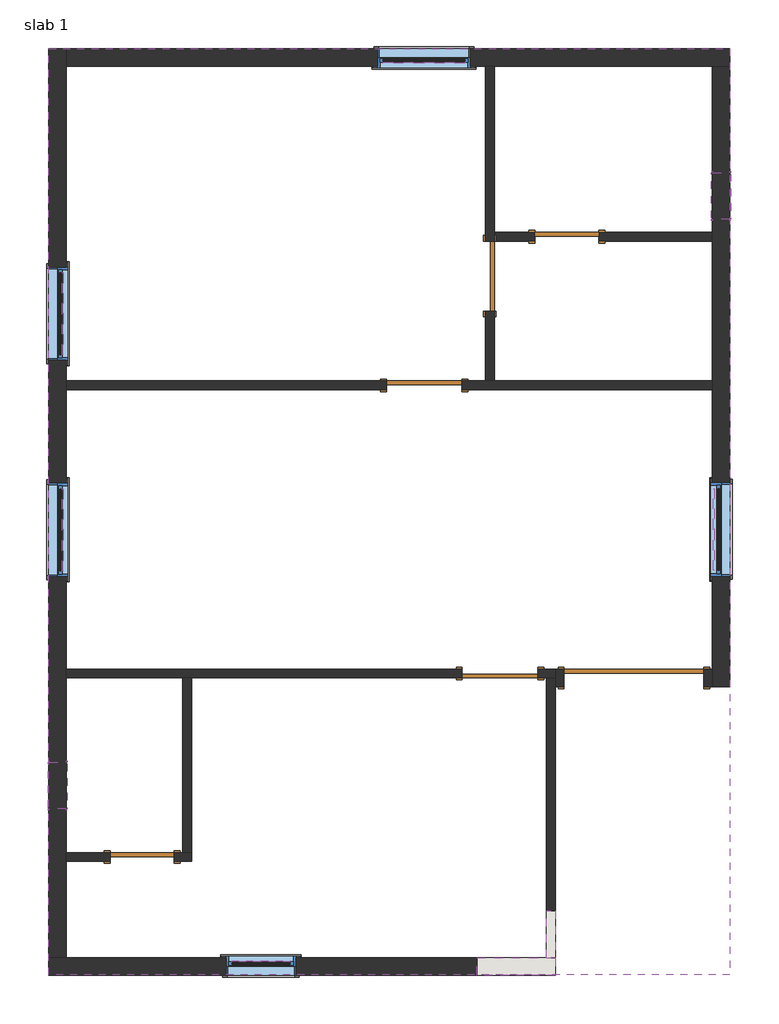
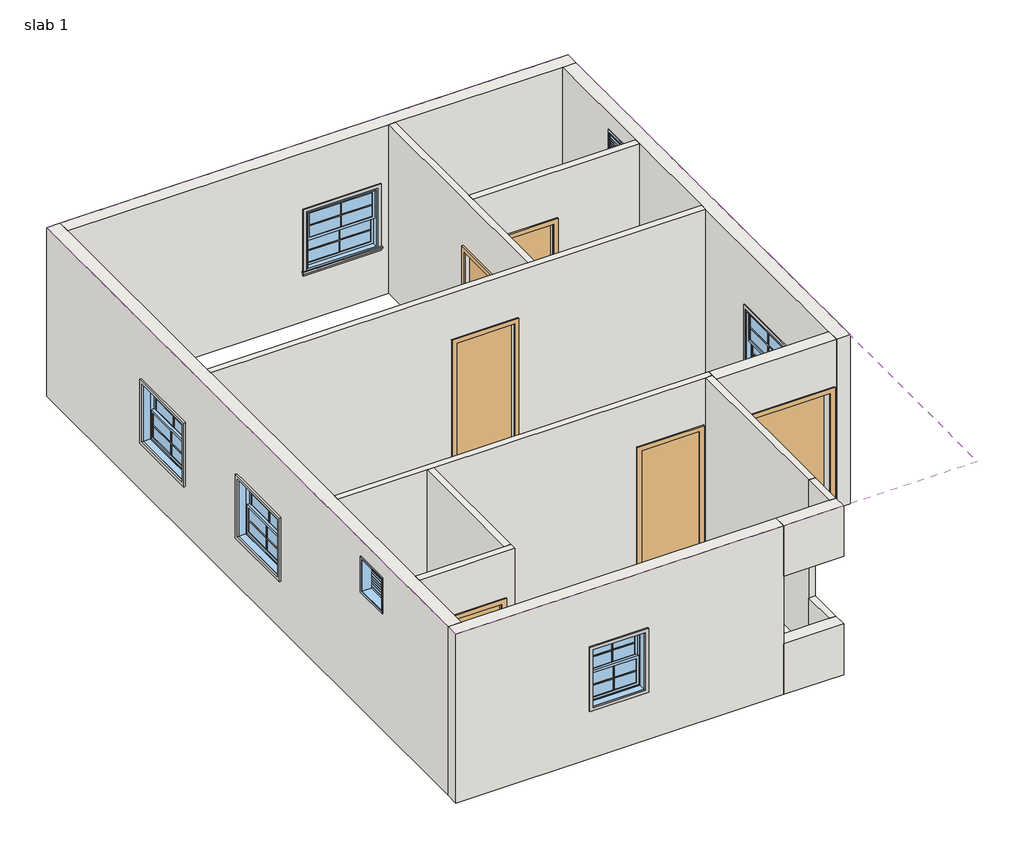
# One storey: 20 proxies, 16 walls, 7 windows, 6 doors, 1 roof.
"""IFC4 building model written with IfcOpenShell, lengths in millimetres."""

from ifc_helpers import new_model, si_unit, frame, origin, place, context, project, spatial, polyline, outline, extrude, faceted_brep, transform, mapped, element, save
from components import muntin_pattern_2x2_muntin_pattern_2x2_0e62f131, muntin_pattern_2x2_muntin_pattern_2x2_8b3f23e7, trim_window_exterior_flat_with_sill_1a1a26d5, trim_window_exterior_flat_with_sill_f44f30ad, trim_window_interior_flat_picture_frame_dc353545, trim_window_interior_flat_picture_frame_1dce1945, single_flush_3_d_305aa2a5, single_flush_6_d_bd5e0b13, single_flush_d2_19300210, single_flush_d3_0217d254, single_flush_d3_43e5c869, single_flush_d4_f1814d11, window_double_hung_3_w_bcdebe7f, window_double_hung_4_eadb0177, window_louvers_2_f2d8fef0

model = new_model("IFC4")

# Units and contexts
model_context = context("Model", 3, world=origin())
ifc_project = project(units=[si_unit("LENGTHUNIT", "METRE", prefix="MILLI")], contexts=[model_context])

# Site, building, storey
site = spatial("IfcSite", under=ifc_project)
building = spatial("IfcBuilding", under=site)
storey = spatial("IfcBuildingStorey", under=building, Name="slab 1", Elevation=3200.4)

# Proxies
placement = place(None, origin())
muntin_pattern_2x2_muntin_pattern_2x2_shape = muntin_pattern_2x2_muntin_pattern_2x2_0e62f131(model_context)
element("IfcBuildingElementProxy", 1, Name="Muntin Pattern_2x2 : Muntin Pattern_2x2", ObjectType="Muntin Pattern_2x2 : Muntin Pattern_2x2", at=placement, inside=storey, context=model_context, shape_type="MappedRepresentation", body=[
    mapped(muntin_pattern_2x2_muntin_pattern_2x2_shape, transform((-20143.9268374, -3803.3341109, 4670.425), x_axis=(1.0, 0.0, 0.0), y_axis=(0.0, 1.0, 0.0), z_axis=(0.0, 0.0, 1.0))),
])
element("IfcBuildingElementProxy", 2, Name="Muntin Pattern_2x2 : Muntin Pattern_2x2", ObjectType="Muntin Pattern_2x2 : Muntin Pattern_2x2", at=placement, inside=storey, context=model_context, shape_type="MappedRepresentation", body=[
    mapped(muntin_pattern_2x2_muntin_pattern_2x2_shape, transform((-20143.9268374, -3847.7841109, 4191.0), x_axis=(1.0, 0.0, 0.0), y_axis=(0.0, 1.0, 0.0), z_axis=(0.0, 0.0, 1.0))),
])
muntin_pattern_2x2_muntin_pattern_2x2_2_shape = muntin_pattern_2x2_muntin_pattern_2x2_8b3f23e7(model_context)
element("IfcBuildingElementProxy", 3, Name="Muntin Pattern_2x2 : Muntin Pattern_2x2", ObjectType="Muntin Pattern_2x2 : Muntin Pattern_2x2", at=placement, inside=storey, context=model_context, shape_type="MappedRepresentation", body=[
    mapped(muntin_pattern_2x2_muntin_pattern_2x2_2_shape, transform((-14197.9649593, 1832.2908097, 4670.425), x_axis=(0.0, 1.0, 0.0), y_axis=(-1.0, 0.0, 0.0), z_axis=(0.0, 0.0, 1.0))),
])
element("IfcBuildingElementProxy", 4, Name="Muntin Pattern_2x2 : Muntin Pattern_2x2", ObjectType="Muntin Pattern_2x2 : Muntin Pattern_2x2", at=placement, inside=storey, context=model_context, shape_type="MappedRepresentation", body=[
    mapped(muntin_pattern_2x2_muntin_pattern_2x2_2_shape, transform((-14153.5149593, 1832.2908097, 4191.0), x_axis=(0.0, 1.0, 0.0), y_axis=(-1.0, 0.0, 0.0), z_axis=(0.0, 0.0, 1.0))),
])
element("IfcBuildingElementProxy", 5, Name="Muntin Pattern_2x2 : Muntin Pattern_2x2", ObjectType="Muntin Pattern_2x2 : Muntin Pattern_2x2", at=placement, inside=storey, context=model_context, shape_type="MappedRepresentation", body=[
    mapped(muntin_pattern_2x2_muntin_pattern_2x2_2_shape, transform((-18009.6223612, 7925.1158098, 4670.425), x_axis=(-1.0, 0.0, 0.0), y_axis=(0.0, -1.0, 0.0), z_axis=(0.0, 0.0, 1.0))),
])
element("IfcBuildingElementProxy", 6, Name="Muntin Pattern_2x2 : Muntin Pattern_2x2", ObjectType="Muntin Pattern_2x2 : Muntin Pattern_2x2", at=placement, inside=storey, context=model_context, shape_type="MappedRepresentation", body=[
    mapped(muntin_pattern_2x2_muntin_pattern_2x2_2_shape, transform((-18009.6223612, 7969.5658098, 4191.0), x_axis=(-1.0, 0.0, 0.0), y_axis=(0.0, -1.0, 0.0), z_axis=(0.0, 0.0, 1.0))),
])
element("IfcBuildingElementProxy", 7, Name="Muntin Pattern_2x2 : Muntin Pattern_2x2", ObjectType="Muntin Pattern_2x2 : Muntin Pattern_2x2", at=placement, inside=storey, context=model_context, shape_type="MappedRepresentation", body=[
    mapped(muntin_pattern_2x2_muntin_pattern_2x2_2_shape, transform((-22726.0149593, 4654.6269753, 4670.425), x_axis=(0.0, -1.0, 0.0), y_axis=(1.0, 0.0, 0.0), z_axis=(0.0, 0.0, 1.0))),
])
element("IfcBuildingElementProxy", 8, Name="Muntin Pattern_2x2 : Muntin Pattern_2x2", ObjectType="Muntin Pattern_2x2 : Muntin Pattern_2x2", at=placement, inside=storey, context=model_context, shape_type="MappedRepresentation", body=[
    mapped(muntin_pattern_2x2_muntin_pattern_2x2_2_shape, transform((-22770.4649593, 4654.6269753, 4191.0), x_axis=(0.0, -1.0, 0.0), y_axis=(1.0, 0.0, 0.0), z_axis=(0.0, 0.0, 1.0))),
])
element("IfcBuildingElementProxy", 9, Name="Muntin Pattern_2x2 : Muntin Pattern_2x2", ObjectType="Muntin Pattern_2x2 : Muntin Pattern_2x2", at=placement, inside=storey, context=model_context, shape_type="MappedRepresentation", body=[
    mapped(muntin_pattern_2x2_muntin_pattern_2x2_2_shape, transform((-22726.0149593, 1826.6103038, 4670.425), x_axis=(0.0, -1.0, 0.0), y_axis=(1.0, 0.0, 0.0), z_axis=(0.0, 0.0, 1.0))),
])
element("IfcBuildingElementProxy", 10, Name="Muntin Pattern_2x2 : Muntin Pattern_2x2", ObjectType="Muntin Pattern_2x2 : Muntin Pattern_2x2", at=placement, inside=storey, context=model_context, shape_type="MappedRepresentation", body=[
    mapped(muntin_pattern_2x2_muntin_pattern_2x2_2_shape, transform((-22770.4649593, 1826.6103038, 4191.0), x_axis=(0.0, -1.0, 0.0), y_axis=(1.0, 0.0, 0.0), z_axis=(0.0, 0.0, 1.0))),
])
trim_window_exterior_flat_with_sill_shape = trim_window_exterior_flat_with_sill_1a1a26d5(model_context)
element("IfcBuildingElementProxy", 11, Name="Trim-Window-Exterior-Flat : with Sill", ObjectType="Trim-Window-Exterior-Flat : with Sill", at=placement, inside=storey, context=model_context, shape_type="MappedRepresentation", body=[
    mapped(trim_window_exterior_flat_with_sill_shape, transform((-20143.9268374, -3768.4091109, 5181.6), x_axis=(-1.0, 0.0, 0.0), y_axis=(0.0, 0.0, 1.0), z_axis=(0.0, 1.0, 0.0))),
])
trim_window_exterior_flat_with_sill_2_shape = trim_window_exterior_flat_with_sill_f44f30ad(model_context)
element("IfcBuildingElementProxy", 12, Name="Trim-Window-Exterior-Flat : with Sill", ObjectType="Trim-Window-Exterior-Flat : with Sill", at=placement, inside=storey, context=model_context, shape_type="MappedRepresentation", body=[
    mapped(trim_window_exterior_flat_with_sill_2_shape, transform((-14232.8899593, 1832.2908097, 5181.6), x_axis=(0.0, -1.0, 0.0), y_axis=(0.0, 0.0, 1.0), z_axis=(-1.0, 0.0, 0.0))),
])
element("IfcBuildingElementProxy", 13, Name="Trim-Window-Exterior-Flat : with Sill", ObjectType="Trim-Window-Exterior-Flat : with Sill", at=placement, inside=storey, context=model_context, shape_type="MappedRepresentation", body=[
    mapped(trim_window_exterior_flat_with_sill_2_shape, transform((-18009.6223612, 7890.1908098, 5181.6), x_axis=(1.0, 0.0, 0.0), y_axis=(0.0, 0.0, 1.0), z_axis=(0.0, -1.0, 0.0))),
])
element("IfcBuildingElementProxy", 14, Name="Trim-Window-Exterior-Flat : with Sill", ObjectType="Trim-Window-Exterior-Flat : with Sill", at=placement, inside=storey, context=model_context, shape_type="MappedRepresentation", body=[
    mapped(trim_window_exterior_flat_with_sill_2_shape, transform((-22691.0899593, 4654.6269753, 5181.6), x_axis=(0.0, 1.0, 0.0), y_axis=(0.0, 0.0, 1.0), z_axis=(1.0, 0.0, 0.0))),
])
element("IfcBuildingElementProxy", 15, Name="Trim-Window-Exterior-Flat : with Sill", ObjectType="Trim-Window-Exterior-Flat : with Sill", at=placement, inside=storey, context=model_context, shape_type="MappedRepresentation", body=[
    mapped(trim_window_exterior_flat_with_sill_2_shape, transform((-22691.0899593, 1826.6103038, 5181.6), x_axis=(0.0, 1.0, 0.0), y_axis=(0.0, 0.0, 1.0), z_axis=(1.0, 0.0, 0.0))),
])
trim_window_interior_flat_picture_frame_shape = trim_window_interior_flat_picture_frame_dc353545(model_context)
element("IfcBuildingElementProxy", 16, Name="Trim-Window-Interior-Flat : Picture Frame", ObjectType="Trim-Window-Interior-Flat : Picture Frame", at=placement, inside=storey, context=model_context, shape_type="MappedRepresentation", body=[
    mapped(trim_window_interior_flat_picture_frame_shape, transform((-20143.9268374, -3997.0091109, 5181.6), x_axis=(1.0, 0.0, 0.0), y_axis=(0.0, 0.0, 1.0), z_axis=(0.0, -1.0, 0.0))),
])
trim_window_interior_flat_picture_frame_2_shape = trim_window_interior_flat_picture_frame_1dce1945(model_context)
element("IfcBuildingElementProxy", 17, Name="Trim-Window-Interior-Flat : Picture Frame", ObjectType="Trim-Window-Interior-Flat : Picture Frame", at=placement, inside=storey, context=model_context, shape_type="MappedRepresentation", body=[
    mapped(trim_window_interior_flat_picture_frame_2_shape, transform((-14004.2899593, 1832.2908097, 5181.6), x_axis=(0.0, 1.0, 0.0), y_axis=(0.0, 0.0, 1.0), z_axis=(1.0, 0.0, 0.0))),
])
element("IfcBuildingElementProxy", 18, Name="Trim-Window-Interior-Flat : Picture Frame", ObjectType="Trim-Window-Interior-Flat : Picture Frame", at=placement, inside=storey, context=model_context, shape_type="MappedRepresentation", body=[
    mapped(trim_window_interior_flat_picture_frame_2_shape, transform((-18009.6223612, 8118.7908098, 5181.6), x_axis=(-1.0, 0.0, 0.0), y_axis=(0.0, 0.0, 1.0), z_axis=(0.0, 1.0, 0.0))),
])
element("IfcBuildingElementProxy", 19, Name="Trim-Window-Interior-Flat : Picture Frame", ObjectType="Trim-Window-Interior-Flat : Picture Frame", at=placement, inside=storey, context=model_context, shape_type="MappedRepresentation", body=[
    mapped(trim_window_interior_flat_picture_frame_2_shape, transform((-22919.6899593, 4654.6269753, 5181.6), x_axis=(0.0, -1.0, 0.0), y_axis=(0.0, 0.0, 1.0), z_axis=(-1.0, 0.0, 0.0))),
])
element("IfcBuildingElementProxy", 20, Name="Trim-Window-Interior-Flat : Picture Frame", ObjectType="Trim-Window-Interior-Flat : Picture Frame", at=placement, inside=storey, context=model_context, shape_type="MappedRepresentation", body=[
    mapped(trim_window_interior_flat_picture_frame_2_shape, transform((-22919.6899593, 1826.6103038, 5181.6), x_axis=(0.0, -1.0, 0.0), y_axis=(0.0, 0.0, 1.0), z_axis=(-1.0, 0.0, 0.0))),
])

# Doors
single_flush_3_d_shape = single_flush_3_d_305aa2a5(model_context)
element("IfcDoor", 21, ObjectType="Single-Flush : 3'd", at=placement, inside=storey, context=model_context, shape_type="MappedRepresentation", body=[
    mapped(single_flush_3_d_shape, transform((-17147.5399593, 5146.9908098, 3200.4), x_axis=(0.0, 1.0, 0.0), y_axis=(-1.0, 0.0, 0.0), z_axis=(0.0, 0.0, 1.0))),
])
single_flush_6_d_shape = single_flush_6_d_bd5e0b13(model_context)
element("IfcDoor", 22, ObjectType="Single-Flush : 6'd", at=placement, inside=storey, context=model_context, shape_type="MappedRepresentation", body=[
    mapped(single_flush_6_d_shape, transform((-15261.5899593, -110.8091902, 3200.4), x_axis=(1.0, 0.0, 0.0), y_axis=(0.0, 1.0, 0.0), z_axis=(0.0, 0.0, 1.0))),
])
single_flush_d2_shape = single_flush_d2_19300210(model_context)
element("IfcDoor", 23, ObjectType="Single-Flush : d2", at=placement, inside=storey, context=model_context, shape_type="MappedRepresentation", body=[
    mapped(single_flush_d2_shape, transform((-16137.8899593, 5661.3408098, 3200.4), x_axis=(-1.0, 0.0, 0.0), y_axis=(0.0, -1.0, 0.0), z_axis=(0.0, 0.0, 1.0))),
])
single_flush_d3_shape = single_flush_d3_0217d254(model_context)
element("IfcDoor", 24, ObjectType="Single-Flush : d3", at=placement, inside=storey, context=model_context, shape_type="MappedRepresentation", body=[
    mapped(single_flush_d3_shape, transform((-18004.7899593, 3718.2408098, 3200.4), x_axis=(1.0, 0.0, 0.0), y_axis=(0.0, 1.0, 0.0), z_axis=(0.0, 0.0, 1.0))),
])
single_flush_d3_2_shape = single_flush_d3_43e5c869(model_context)
element("IfcDoor", 25, ObjectType="Single-Flush : d3", at=placement, inside=storey, context=model_context, shape_type="MappedRepresentation", body=[
    mapped(single_flush_d3_2_shape, transform((-17014.1899593, -53.6591902, 3200.4), x_axis=(1.0, 0.0, 0.0), y_axis=(0.0, 1.0, 0.0), z_axis=(0.0, 0.0, 1.0))),
])
single_flush_d4_shape = single_flush_d4_f1814d11(model_context)
element("IfcDoor", 26, ObjectType="Single-Flush : d4", at=placement, inside=storey, context=model_context, shape_type="MappedRepresentation", body=[
    mapped(single_flush_d4_shape, transform((-21700.4899593, -2453.9591902, 3200.4), x_axis=(1.0, 0.0, 0.0), y_axis=(0.0, 1.0, 0.0), z_axis=(0.0, 0.0, 1.0))),
])

# Roof
element("IfcRoof", 27, ObjectType="6\" slab", at=placement, inside=storey, context=model_context, shape_type="SweptSolid", body=[
    extrude(outline(polyline([(-22919.6899593, 8118.7908098), (-14004.2899593, 8118.7908098), (-14004.2899593, -3997.0091109), (-22919.6899593, -3997.0091109), (-22919.6899593, 8118.7908098)])), frame((0.0, 0.0, 6248.4), z_axis=(0.0, 0.0, 1.0), x_axis=(1.0, 0.0, 0.0)), (0.0, 0.0, 1.0), 152.4),
])

# Walls
element("IfcWall", 28, ObjectType="4.5\" w", at=placement, inside=storey, context=model_context, shape_type="Brep", body=[
    faceted_brep([(-17509.4899593, 3661.0908098, 5334.0), (-17509.4899593, 3661.0908098, 3200.4), (-14232.8899593, 3661.0908098, 3200.4), (-14232.8899593, 3661.0908098, 6248.4), (-22691.0899593, 3661.0908098, 6248.4), (-22691.0899593, 3661.0908098, 3200.4), (-18500.0899593, 3661.0908098, 3200.4), (-18500.0899593, 3661.0908098, 5334.0), (-14232.8899593, 3775.3908098, 3200.4), (-17090.3899593, 3775.3908098, 3200.4), (-17204.6899593, 3775.3908098, 3200.4), (-17509.4899593, 3775.3908098, 3200.4), (-17509.4899593, 3775.3908098, 5334.0), (-18500.0899593, 3775.3908098, 5334.0), (-18500.0899593, 3775.3908098, 3200.4), (-22691.0899593, 3775.3908098, 3200.4), (-22691.0899593, 3775.3908098, 6248.4), (-17204.6899593, 3775.3908098, 6248.4), (-17090.3899593, 3775.3908098, 6248.4), (-14232.8899593, 3775.3908098, 6248.4)], [[[0, 1, 2, 3, 4, 5, 6, 7]], [[8, 9, 10, 11, 12, 13, 14, 15, 16, 17, 18, 19]], [[6, 5, 15, 14]], [[2, 1, 11, 10, 9, 8]], [[4, 3, 19, 18, 17, 16]], [[5, 4, 16, 15]], [[3, 2, 8, 19]], [[12, 11, 1, 0]], [[13, 12, 0, 7]], [[14, 13, 7, 6]]]),
])
element("IfcWall", 29, ObjectType="4.5\" w", at=placement, inside=storey, context=model_context, shape_type="Brep", body=[
    faceted_brep([(-17204.6899593, 7890.1908098, 3200.4), (-17204.6899593, 5604.1908098, 3200.4), (-17204.6899593, 5604.1908098, 5334.0), (-17204.6899593, 4689.7908098, 5334.0), (-17204.6899593, 4689.7908098, 3200.4), (-17204.6899593, 3775.3908098, 3200.4), (-17204.6899593, 3775.3908098, 6248.4), (-17204.6899593, 7890.1908098, 6248.4), (-17090.3899593, 5604.1908098, 5334.0), (-17090.3899593, 5604.1908098, 3200.4), (-17090.3899593, 5718.4908098, 3200.4), (-17090.3899593, 7890.1908098, 3200.4), (-17090.3899593, 7890.1908098, 6248.4), (-17090.3899593, 5718.4908098, 6248.4), (-17090.3899593, 5604.1908098, 6248.4), (-17090.3899593, 3775.3908098, 6248.4), (-17090.3899593, 3775.3908098, 3200.4), (-17090.3899593, 4689.7908098, 3200.4), (-17090.3899593, 4689.7908098, 5334.0)], [[[0, 1, 2, 3, 4, 5, 6, 7]], [[8, 9, 10, 11, 12, 13, 14, 15, 16, 17, 18]], [[17, 16, 5, 4]], [[11, 10, 9, 1, 0]], [[7, 6, 15, 14, 13, 12]], [[0, 7, 12, 11]], [[6, 5, 16, 15]], [[2, 1, 9, 8]], [[3, 2, 8, 18]], [[4, 3, 18, 17]]]),
])
element("IfcWall", 30, ObjectType="4.5\" w", at=placement, inside=storey, context=model_context, shape_type="Brep", body=[
    faceted_brep([(-16556.9899593, 5718.4908098, 5334.0), (-16556.9899593, 5718.4908098, 3200.4), (-17090.3899593, 5718.4908098, 3200.4), (-17090.3899593, 5718.4908098, 6248.4), (-14232.8899593, 5718.4908098, 6248.4), (-14232.8899593, 5718.4908098, 3200.4), (-15718.7899593, 5718.4908098, 3200.4), (-15718.7899593, 5718.4908098, 5334.0), (-17090.3899593, 5604.1908098, 3200.4), (-16556.9899593, 5604.1908098, 3200.4), (-16556.9899593, 5604.1908098, 5334.0), (-15718.7899593, 5604.1908098, 5334.0), (-15718.7899593, 5604.1908098, 3200.4), (-14232.8899593, 5604.1908098, 3200.4), (-14232.8899593, 5604.1908098, 6248.4), (-17090.3899593, 5604.1908098, 6248.4), (-17090.3899593, 5604.1908098, 5334.0)], [[[0, 1, 2, 3, 4, 5, 6, 7]], [[8, 9, 10, 11, 12, 13, 14, 15, 16]], [[6, 5, 13, 12]], [[2, 1, 9, 8]], [[4, 3, 15, 14]], [[5, 4, 14, 13]], [[3, 2, 8, 16, 15]], [[10, 9, 1, 0]], [[11, 10, 0, 7]], [[12, 11, 7, 6]]]),
])
element("IfcWall", 31, ObjectType="4.5\" w", at=placement, inside=storey, context=model_context, shape_type="Brep", body=[
    faceted_brep([(-16518.8899593, -110.8091902, 5334.0), (-16518.8899593, -110.8091902, 3200.4), (-16404.5899587, -110.8091902, 3200.4), (-16290.2899587, -110.8091902, 3200.4), (-16290.2899587, -110.8091902, 6248.4), (-16404.5899587, -110.8091902, 6248.4), (-21052.7899593, -110.8091902, 6248.4), (-21167.0899593, -110.8091902, 6248.4), (-22691.0899593, -110.8091902, 6248.4), (-22691.0899593, -110.8091902, 3200.4), (-21167.0899593, -110.8091902, 3200.4), (-21052.7899593, -110.8091902, 3200.4), (-17509.4899593, -110.8091902, 3200.4), (-17509.4899593, -110.8091902, 5334.0), (-16290.2899587, 3.4908098, 3200.4), (-16518.8899593, 3.4908098, 3200.4), (-16518.8899593, 3.4908098, 5334.0), (-17509.4899593, 3.4908098, 5334.0), (-17509.4899593, 3.4908098, 3200.4), (-22691.0899593, 3.4908098, 3200.4), (-22691.0899593, 3.4908098, 6248.4), (-16290.2899587, 3.4908098, 6248.4)], [[[0, 1, 2, 3, 4, 5, 6, 7, 8, 9, 10, 11, 12, 13]], [[14, 15, 16, 17, 18, 19, 20, 21]], [[3, 2, 1, 15, 14]], [[12, 11, 10, 9, 19, 18]], [[8, 7, 6, 5, 4, 21, 20]], [[9, 8, 20, 19]], [[4, 3, 14, 21]], [[16, 15, 1, 0]], [[17, 16, 0, 13]], [[18, 17, 13, 12]]]),
])
element("IfcWall", 32, ObjectType="4.5\" w", at=placement, inside=storey, context=model_context, shape_type="Brep", body=[
    faceted_brep([(-16404.5899587, -110.8091902, 3200.4), (-16404.5899587, -3158.8091902, 3200.4), (-16404.5899587, -3158.8091902, 4114.8), (-16404.5899587, -3158.8091902, 5334.0), (-16404.5899587, -3158.8091902, 6248.4), (-16404.5899587, -110.8091902, 6248.4), (-16290.2899587, -110.8091902, 3200.4), (-16290.2899587, -110.8091902, 6248.4), (-16290.2899587, -225.1091902, 6248.4), (-16290.2899587, -3158.8091902, 6248.4), (-16290.2899587, -3158.8091902, 5334.0), (-16290.2899587, -3158.8091902, 4114.8), (-16290.2899587, -3158.8091902, 3200.4), (-16290.2899587, -225.1091902, 3200.4)], [[[0, 1, 2, 3, 4, 5]], [[6, 7, 8, 9, 10, 11, 12, 13]], [[1, 0, 6, 13, 12]], [[5, 4, 9, 8, 7]], [[0, 5, 7, 6]], [[1, 12, 11, 10, 9, 4, 3, 2]]]),
])
element("IfcWall", 33, ObjectType="4.5\" w", at=placement, inside=storey, context=model_context, shape_type="Brep", body=[
    faceted_brep([(-21281.3899593, -2511.1091902, 5334.0), (-21281.3899593, -2511.1091902, 3200.4), (-21052.7899593, -2511.1091902, 3200.4), (-21052.7899593, -2511.1091902, 6248.4), (-22691.0899593, -2511.1091902, 6248.4), (-22691.0899593, -2511.1091902, 3200.4), (-22119.5899593, -2511.1091902, 3200.4), (-22119.5899593, -2511.1091902, 5334.0), (-21052.7899593, -2396.8091902, 3200.4), (-21167.0899593, -2396.8091902, 3200.4), (-21281.3899593, -2396.8091902, 3200.4), (-21281.3899593, -2396.8091902, 5334.0), (-22119.5899593, -2396.8091902, 5334.0), (-22119.5899593, -2396.8091902, 3200.4), (-22691.0899593, -2396.8091902, 3200.4), (-22691.0899593, -2396.8091902, 6248.4), (-21167.0899593, -2396.8091902, 6248.4), (-21052.7899593, -2396.8091902, 6248.4)], [[[0, 1, 2, 3, 4, 5, 6, 7]], [[8, 9, 10, 11, 12, 13, 14, 15, 16, 17]], [[6, 5, 14, 13]], [[2, 1, 10, 9, 8]], [[4, 3, 17, 16, 15]], [[5, 4, 15, 14]], [[3, 2, 8, 17]], [[11, 10, 1, 0]], [[12, 11, 0, 7]], [[13, 12, 7, 6]]]),
])
element("IfcWall", 34, ObjectType="4.5\" w", at=placement, inside=storey, context=model_context, shape_type="SweptSolid", body=[
    extrude(outline(polyline([(-21052.7899593, -110.8091902), (-21052.7899593, -2396.8091902), (-21167.0899593, -2396.8091902), (-21167.0899593, -110.8091902), (-21052.7899593, -110.8091902)])), frame((0.0, 0.0, 3200.4), z_axis=(0.0, 0.0, 1.0), x_axis=(1.0, 0.0, 0.0)), (0.0, 0.0, 1.0), 3048.0),
])
element("IfcWall", 35, ObjectType="4.5\" w 2", at=placement, inside=storey, context=model_context, shape_type="SweptSolid", body=[
    extrude(outline(polyline([(-16404.5899587, -3768.4091109), (-16404.5899587, -3158.8091902), (-16290.2899587, -3158.8091902), (-16290.2899587, -3768.4091109), (-16404.5899587, -3768.4091109)])), frame((0.0, 0.0, 3200.4), z_axis=(0.0, 0.0, 1.0), x_axis=(1.0, 0.0, 0.0)), (0.0, 0.0, 1.0), 914.4),
])
element("IfcWall", 36, ObjectType="4.5\" w 2", at=placement, inside=storey, context=model_context, shape_type="SweptSolid", body=[
    extrude(outline(polyline([(-16404.5899587, -3768.4091109), (-16404.5899587, -3158.8091902), (-16290.2899587, -3158.8091902), (-16290.2899587, -3768.4091109), (-16404.5899587, -3768.4091109)])), frame((0.0, 0.0, 5334.0), z_axis=(0.0, 0.0, 1.0), x_axis=(1.0, 0.0, 0.0)), (0.0, 0.0, 1.0), 914.4),
])
element("IfcWall", 37, ObjectType="9\" w", at=placement, inside=storey, context=model_context, shape_type="Brep", body=[
    faceted_brep([(-17318.9899593, -3768.4091109, 6248.4), (-17318.9899593, -3768.4091109, 5334.0), (-17318.9899593, -3768.4091109, 4114.8), (-17318.9899593, -3768.4091109, 3200.4), (-22691.0899593, -3768.4091109, 3200.4), (-22919.6899593, -3768.4091109, 3200.4), (-22919.6899593, -3768.4091109, 6248.4), (-22691.0899593, -3768.4091109, 6248.4), (-20601.1268374, -3768.4091109, 5181.6), (-20601.1268374, -3768.4091109, 4114.8), (-19686.7268374, -3768.4091109, 4114.8), (-19686.7268374, -3768.4091109, 5181.6), (-17318.9899593, -3997.0091109, 3200.4), (-17318.9899593, -3997.0091109, 4114.8), (-17318.9899593, -3997.0091109, 5334.0), (-17318.9899593, -3997.0091109, 6248.4), (-22919.6899593, -3997.0091109, 6248.4), (-22919.6899593, -3997.0091109, 3200.4), (-20601.1268374, -3997.0091109, 5181.6), (-19686.7268374, -3997.0091109, 5181.6), (-19686.7268374, -3997.0091109, 4114.8), (-20601.1268374, -3997.0091109, 4114.8)], [[[0, 1, 2, 3, 4, 5, 6, 7], [8, 9, 10, 11]], [[12, 13, 14, 15, 16, 17], [18, 19, 20, 21]], [[5, 4, 3, 12, 17]], [[0, 7, 6, 16, 15]], [[6, 5, 17, 16]], [[9, 8, 18, 21]], [[10, 9, 21, 20]], [[11, 10, 20, 19]], [[8, 11, 19, 18]], [[0, 15, 14, 13, 12, 3, 2, 1]]]),
])
element("IfcWall", 38, ObjectType="9\" w", at=placement, inside=storey, context=model_context, shape_type="Brep", body=[
    faceted_brep([(-22691.0899593, -3768.4091109, 3200.4), (-22691.0899593, -2511.1091902, 3200.4), (-22691.0899593, -2396.8091902, 3200.4), (-22691.0899593, -110.8091902, 3200.4), (-22691.0899593, 3.4908098, 3200.4), (-22691.0899593, 3661.0908098, 3200.4), (-22691.0899593, 3775.3908098, 3200.4), (-22691.0899593, 7890.1908098, 3200.4), (-22691.0899593, 8118.7908098, 3200.4), (-22691.0899593, 8118.7908098, 6248.4), (-22691.0899593, 7890.1908098, 6248.4), (-22691.0899593, 3775.3908098, 6248.4), (-22691.0899593, 3661.0908098, 6248.4), (-22691.0899593, 3.4908098, 6248.4), (-22691.0899593, -110.8091902, 6248.4), (-22691.0899593, -2396.8091902, 6248.4), (-22691.0899593, -2511.1091902, 6248.4), (-22691.0899593, -3768.4091109, 6248.4), (-22691.0899593, 5264.2269753, 5181.6), (-22691.0899593, 5264.2269753, 4114.8), (-22691.0899593, 4045.0269753, 4114.8), (-22691.0899593, 4045.0269753, 5181.6), (-22691.0899593, 2436.2103038, 5181.6), (-22691.0899593, 2436.2103038, 4114.8), (-22691.0899593, 1217.0103038, 4114.8), (-22691.0899593, 1217.0103038, 5181.6), (-22691.0899593, -1215.0396931, 5943.6), (-22691.0899593, -1215.0396931, 5334.0), (-22691.0899593, -1824.6396931, 5334.0), (-22691.0899593, -1824.6396931, 5943.6), (-22919.6899593, -3768.4091109, 3200.4), (-22919.6899593, -3768.4091109, 6248.4), (-22919.6899593, 8118.7908098, 6248.4), (-22919.6899593, 8118.7908098, 3200.4), (-22919.6899593, 5264.2269753, 5181.6), (-22919.6899593, 4045.0269753, 5181.6), (-22919.6899593, 4045.0269753, 4114.8), (-22919.6899593, 5264.2269753, 4114.8), (-22919.6899593, 2436.2103038, 5181.6), (-22919.6899593, 1217.0103038, 5181.6), (-22919.6899593, 1217.0103038, 4114.8), (-22919.6899593, 2436.2103038, 4114.8), (-22919.6899593, -1215.0396931, 5943.6), (-22919.6899593, -1824.6396931, 5943.6), (-22919.6899593, -1824.6396931, 5334.0), (-22919.6899593, -1215.0396931, 5334.0)], [[[0, 1, 2, 3, 4, 5, 6, 7, 8, 9, 10, 11, 12, 13, 14, 15, 16, 17], [18, 19, 20, 21], [22, 23, 24, 25], [26, 27, 28, 29]], [[30, 31, 32, 33], [34, 35, 36, 37], [38, 39, 40, 41], [42, 43, 44, 45]], [[8, 7, 6, 5, 4, 3, 2, 1, 0, 30, 33]], [[17, 16, 15, 14, 13, 12, 11, 10, 9, 32, 31]], [[0, 17, 31, 30]], [[9, 8, 33, 32]], [[19, 18, 34, 37]], [[20, 19, 37, 36]], [[21, 20, 36, 35]], [[18, 21, 35, 34]], [[23, 22, 38, 41]], [[24, 23, 41, 40]], [[25, 24, 40, 39]], [[22, 25, 39, 38]], [[27, 26, 42, 45]], [[28, 27, 45, 44]], [[29, 28, 44, 43]], [[26, 29, 43, 42]]]),
])
element("IfcWall", 39, ObjectType="9\" w", at=placement, inside=storey, context=model_context, shape_type="Brep", body=[
    faceted_brep([(-22691.0899593, 7890.1908098, 3200.4), (-17204.6899593, 7890.1908098, 3200.4), (-17090.3899593, 7890.1908098, 3200.4), (-14232.8899593, 7890.1908098, 3200.4), (-14004.2899593, 7890.1908098, 3200.4), (-14004.2899593, 7890.1908098, 6248.4), (-14232.8899593, 7890.1908098, 6248.4), (-17090.3899593, 7890.1908098, 6248.4), (-17204.6899593, 7890.1908098, 6248.4), (-22691.0899593, 7890.1908098, 6248.4), (-17400.0223612, 7890.1908098, 5181.6), (-17400.0223612, 7890.1908098, 4114.8), (-18619.2223612, 7890.1908098, 4114.8), (-18619.2223612, 7890.1908098, 5181.6), (-22691.0899593, 8118.7908098, 3200.4), (-22691.0899593, 8118.7908098, 6248.4), (-14004.2899593, 8118.7908098, 6248.4), (-14004.2899593, 8118.7908098, 3200.4), (-17400.0223612, 8118.7908098, 5181.6), (-18619.2223612, 8118.7908098, 5181.6), (-18619.2223612, 8118.7908098, 4114.8), (-17400.0223612, 8118.7908098, 4114.8)], [[[0, 1, 2, 3, 4, 5, 6, 7, 8, 9], [10, 11, 12, 13]], [[14, 15, 16, 17], [18, 19, 20, 21]], [[4, 3, 2, 1, 0, 14, 17]], [[9, 8, 7, 6, 5, 16, 15]], [[0, 9, 15, 14]], [[5, 4, 17, 16]], [[11, 10, 18, 21]], [[12, 11, 21, 20]], [[13, 12, 20, 19]], [[10, 13, 19, 18]]]),
])
element("IfcWall", 40, ObjectType="9\" w", at=placement, inside=storey, context=model_context, shape_type="Brep", body=[
    faceted_brep([(-14232.8899593, 7890.1908098, 3200.4), (-14232.8899593, 5718.4908098, 3200.4), (-14232.8899593, 5604.1908098, 3200.4), (-14232.8899593, 3775.3908098, 3200.4), (-14232.8899593, 3661.0908098, 3200.4), (-14232.8899593, 3.4908098, 3200.4), (-14232.8899593, -225.1091902, 3200.4), (-14232.8899593, -225.1091902, 6248.4), (-14232.8899593, 3.4908098, 6248.4), (-14232.8899593, 3661.0908098, 6248.4), (-14232.8899593, 3775.3908098, 6248.4), (-14232.8899593, 5604.1908098, 6248.4), (-14232.8899593, 5718.4908098, 6248.4), (-14232.8899593, 7890.1908098, 6248.4), (-14232.8899593, 1222.6908097, 5181.6), (-14232.8899593, 1222.6908097, 4114.8), (-14232.8899593, 2441.8908097, 4114.8), (-14232.8899593, 2441.8908097, 5181.6), (-14232.8899593, 5889.9408098, 5943.6), (-14232.8899593, 5889.9408098, 5334.0), (-14232.8899593, 6499.5408098, 5334.0), (-14232.8899593, 6499.5408098, 5943.6), (-14004.2899593, 7890.1908098, 3200.4), (-14004.2899593, 7890.1908098, 6248.4), (-14004.2899593, -225.1091902, 6248.4), (-14004.2899593, -225.1091902, 3200.4), (-14004.2899593, 1222.6908097, 5181.6), (-14004.2899593, 2441.8908097, 5181.6), (-14004.2899593, 2441.8908097, 4114.8), (-14004.2899593, 1222.6908097, 4114.8), (-14004.2899593, 5889.9408098, 5943.6), (-14004.2899593, 6499.5408098, 5943.6), (-14004.2899593, 6499.5408098, 5334.0), (-14004.2899593, 5889.9408098, 5334.0)], [[[0, 1, 2, 3, 4, 5, 6, 7, 8, 9, 10, 11, 12, 13], [14, 15, 16, 17], [18, 19, 20, 21]], [[22, 23, 24, 25], [26, 27, 28, 29], [30, 31, 32, 33]], [[6, 5, 4, 3, 2, 1, 0, 22, 25]], [[13, 12, 11, 10, 9, 8, 7, 24, 23]], [[0, 13, 23, 22]], [[7, 6, 25, 24]], [[15, 14, 26, 29]], [[16, 15, 29, 28]], [[17, 16, 28, 27]], [[14, 17, 27, 26]], [[19, 18, 30, 33]], [[20, 19, 33, 32]], [[21, 20, 32, 31]], [[18, 21, 31, 30]]]),
])
element("IfcWall", 41, ObjectType="9\" w", at=placement, inside=storey, context=model_context, shape_type="Brep", body=[
    faceted_brep([(-14232.8899593, 3.4908098, 3200.4), (-14347.1899593, 3.4908098, 3200.4), (-14347.1899593, 3.4908098, 5334.0), (-16175.9899593, 3.4908098, 5334.0), (-16175.9899593, 3.4908098, 3200.4), (-16290.2899587, 3.4908098, 3200.4), (-16290.2899587, 3.4908098, 6248.4), (-14232.8899593, 3.4908098, 6248.4), (-14347.1899593, -225.1091902, 5334.0), (-14347.1899593, -225.1091902, 3200.4), (-14232.8899593, -225.1091902, 3200.4), (-14232.8899593, -225.1091902, 6248.4), (-16290.2899587, -225.1091902, 6248.4), (-16290.2899587, -225.1091902, 3200.4), (-16175.9899593, -225.1091902, 3200.4), (-16175.9899593, -225.1091902, 5334.0), (-16290.2899587, -110.8091902, 3200.4), (-16290.2899587, -110.8091902, 6248.4)], [[[0, 1, 2, 3, 4, 5, 6, 7]], [[8, 9, 10, 11, 12, 13, 14, 15]], [[14, 13, 16, 5, 4]], [[10, 9, 1, 0]], [[7, 6, 17, 12, 11]], [[0, 7, 11, 10]], [[6, 5, 16, 13, 12, 17]], [[2, 1, 9, 8]], [[3, 2, 8, 15]], [[4, 3, 15, 14]]]),
])
element("IfcWall", 42, ObjectType="9\" w 2", at=placement, inside=storey, context=model_context, shape_type="Brep", body=[
    faceted_brep([(-17318.9899593, -3997.0091109, 3200.4), (-16290.2899587, -3997.0091109, 3200.4), (-16290.2899587, -3997.0091109, 4114.8), (-17318.9899593, -3997.0091109, 4114.8), (-17318.9899593, -3768.4091109, 3200.4), (-17318.9899593, -3768.4091109, 4114.8), (-16404.5899587, -3768.4091109, 4114.8), (-16290.2899587, -3768.4091109, 4114.8), (-16290.2899587, -3768.4091109, 3200.4), (-16404.5899587, -3768.4091109, 3200.4)], [[[0, 1, 2, 3]], [[4, 5, 6, 7, 8, 9]], [[1, 0, 4, 9, 8]], [[3, 2, 7, 6, 5]], [[0, 3, 5, 4]], [[2, 1, 8, 7]]]),
])
element("IfcWall", 43, ObjectType="9\" w 2", at=placement, inside=storey, context=model_context, shape_type="Brep", body=[
    faceted_brep([(-17318.9899593, -3997.0091109, 5334.0), (-16290.2899587, -3997.0091109, 5334.0), (-16290.2899587, -3997.0091109, 6248.4), (-17318.9899593, -3997.0091109, 6248.4), (-17318.9899593, -3768.4091109, 5334.0), (-17318.9899593, -3768.4091109, 6248.4), (-16404.5899587, -3768.4091109, 6248.4), (-16290.2899587, -3768.4091109, 6248.4), (-16290.2899587, -3768.4091109, 5334.0), (-16404.5899587, -3768.4091109, 5334.0)], [[[0, 1, 2, 3]], [[4, 5, 6, 7, 8, 9]], [[1, 0, 4, 9, 8]], [[3, 2, 7, 6, 5]], [[0, 3, 5, 4]], [[2, 1, 8, 7]]]),
])

# Windows
window_double_hung_3_w_shape = window_double_hung_3_w_bcdebe7f(model_context)
element("IfcWindow", 44, ObjectType="Window-Double-Hung : 3'w", at=placement, inside=storey, context=model_context, shape_type="MappedRepresentation", body=[
    mapped(window_double_hung_3_w_shape, transform((-20143.9268374, -3882.7091109, 3200.4), x_axis=(1.0, 0.0, 0.0), y_axis=(0.0, 1.0, 0.0), z_axis=(0.0, 0.0, 1.0))),
])
window_double_hung_4_shape = window_double_hung_4_eadb0177(model_context)
element("IfcWindow", 45, ObjectType="Window-Double-Hung : 4'", at=placement, inside=storey, context=model_context, shape_type="MappedRepresentation", body=[
    mapped(window_double_hung_4_shape, transform((-14118.5899593, 1832.2908097, 3200.4), x_axis=(0.0, 1.0, 0.0), y_axis=(-1.0, 0.0, 0.0), z_axis=(0.0, 0.0, 1.0))),
])
element("IfcWindow", 46, ObjectType="Window-Double-Hung : 4'", at=placement, inside=storey, context=model_context, shape_type="MappedRepresentation", body=[
    mapped(window_double_hung_4_shape, transform((-18009.6223612, 8004.4908098, 3200.4), x_axis=(-1.0, 0.0, 0.0), y_axis=(0.0, -1.0, 0.0), z_axis=(0.0, 0.0, 1.0))),
])
element("IfcWindow", 47, ObjectType="Window-Double-Hung : 4'", at=placement, inside=storey, context=model_context, shape_type="MappedRepresentation", body=[
    mapped(window_double_hung_4_shape, transform((-22805.3899593, 4654.6269753, 3200.4), x_axis=(0.0, -1.0, 0.0), y_axis=(1.0, 0.0, 0.0), z_axis=(0.0, 0.0, 1.0))),
])
element("IfcWindow", 48, ObjectType="Window-Double-Hung : 4'", at=placement, inside=storey, context=model_context, shape_type="MappedRepresentation", body=[
    mapped(window_double_hung_4_shape, transform((-22805.3899593, 1826.6103038, 3200.4), x_axis=(0.0, -1.0, 0.0), y_axis=(1.0, 0.0, 0.0), z_axis=(0.0, 0.0, 1.0))),
])
window_louvers_2_shape = window_louvers_2_f2d8fef0(model_context)
element("IfcWindow", 49, ObjectType="Window-Louvers : 2'", at=placement, inside=storey, context=model_context, shape_type="MappedRepresentation", body=[
    mapped(window_louvers_2_shape, transform((-22799.0399593, -1519.8396931, 4419.6), x_axis=(0.0, -1.0, 0.0), y_axis=(1.0, 0.0, 0.0), z_axis=(0.0, 0.0, 1.0))),
])
element("IfcWindow", 50, ObjectType="Window-Louvers : 2'", at=placement, inside=storey, context=model_context, shape_type="MappedRepresentation", body=[
    mapped(window_louvers_2_shape, transform((-14124.9399593, 6194.7408098, 4419.6), x_axis=(0.0, 1.0, 0.0), y_axis=(-1.0, 0.0, 0.0), z_axis=(0.0, 0.0, 1.0))),
])

save(model, "model.ifc")

# Revit data of these elements
# Type "Muntin Pattern_2x2 : Muntin Pattern_2x2"
#   Width [instance default] = 4' - 0"
#   Thickness = 0' - 0 1/2"
#   Height [instance default] = 4' - 0"
#   Distance = 0' - 0 3/4"
#   Interior Material [instance default] = none
#   Exterior Material [instance default] = none
#   Default Elevation = 0
# Type "Trim-Window-Exterior-Flat : with Sill"
#   Trim Width = 0' - 2 1/4"
#   Trim Thickness_Picture Frame = 0' - 1 1/4"
#   Trim Thickness_with Sill = 0' - 0 3/4"
#   Sill Thickness = 0' - 1 1/4"
#   Opening Width [instance default] = 2' - 0"
#   Opening Height [instance default] = 3' - 0"
#   Default Elevation = 4' - 0"
#   Sill = yes
#   Picture Frame = no
#   Trim Material [instance default] = none
# Type "Trim-Window-Interior-Flat : Picture Frame"
#   Trim Thickness_Picture Frame = 0' - 1 1/4"
#   Trim Width = 0' - 2 1/4"
#   Trim Thickness_with Sill = 0' - 0 3/4"
#   Sill Thickness = 0' - 1 1/4"
#   Opening Width [instance default] = 2' - 0"
#   Opening Height [instance default] = 3' - 0"
#   Default Elevation = 4' - 0"
#   Sill = no
#   Picture Frame = yes
#   Trim Material [instance default] = none
# Type "Single-Flush : 3'd"
#   Type Mark = "13"
#   Construction Type Id = "MDOOR"
#   Assembly Code = "C1020"
#   Analytic Construction = "Metal"
#   Thickness = 0' - 2"
#   Heat Transfer Coefficient (U) = 0.651978 BTU/(h·ft²·°F)
#   Height = 7' - 0"
#   Trim Projection Ext = 0' - 1"
#   Trim Projection Int = 0' - 1"
#   Trim Width = 0' - 3"
#   Width = 3' - 0"
#   Define Thermal Properties by = 1
#   Door Material = Door - Panel
#   Frame Material = Door - Frame
#   Visual Light Transmittance = 0
#   Solar Heat Gain Coefficient = 0
#   Function = (empty or 0)
#   Wall Closure = (empty or 0)
# Type "Single-Flush : 6'd"
#   Type Mark = "14"
#   Construction Type Id = "MDOOR"
#   Assembly Code = "C1020"
#   Analytic Construction = "Metal"
#   Thickness = 0' - 2"
#   Heat Transfer Coefficient (U) = 0.651978 BTU/(h·ft²·°F)
#   Height = 7' - 0"
#   Trim Projection Ext = 0' - 1"
#   Trim Projection Int = 0' - 1"
#   Trim Width = 0' - 3"
#   Width = 6' - 0"
#   Define Thermal Properties by = 1
#   Door Material = Door - Panel
#   Frame Material = Door - Frame
#   Visual Light Transmittance = 0
#   Solar Heat Gain Coefficient = 0
#   Function = (empty or 0)
#   Wall Closure = (empty or 0)
# Type "Single-Flush : d2"
#   Type Mark = "9"
#   Construction Type Id = "MDOOR"
#   Assembly Code = "C1020"
#   Analytic Construction = "Metal"
#   Thickness = 0' - 2"
#   Heat Transfer Coefficient (U) = 0.651978 BTU/(h·ft²·°F)
#   Height = 7' - 0"
#   Trim Projection Ext = 0' - 1"
#   Trim Projection Int = 0' - 1"
#   Trim Width = 0' - 3"
#   Width = 2' - 9"
#   Define Thermal Properties by = 1
#   Door Material = Door - Panel
#   Frame Material = Door - Frame
#   Visual Light Transmittance = 0
#   Solar Heat Gain Coefficient = 0
#   Function = (empty or 0)
#   Wall Closure = (empty or 0)
# Type "Single-Flush : d3"
#   Type Mark = "10"
#   Construction Type Id = "MDOOR"
#   Assembly Code = "C1020"
#   Analytic Construction = "Metal"
#   Thickness = 0' - 2"
#   Heat Transfer Coefficient (U) = 0.651978 BTU/(h·ft²·°F)
#   Height = 7' - 0"
#   Trim Projection Ext = 0' - 1"
#   Trim Projection Int = 0' - 1"
#   Trim Width = 0' - 3"
#   Width = 3' - 3"
#   Define Thermal Properties by = 1
#   Door Material = Door - Panel
#   Frame Material = Door - Frame
#   Visual Light Transmittance = 0
#   Solar Heat Gain Coefficient = 0
#   Function = (empty or 0)
#   Wall Closure = (empty or 0)
# Type "Single-Flush : d4"
#   Type Mark = "11"
#   Construction Type Id = "MDOOR"
#   Assembly Code = "C1020"
#   Analytic Construction = "Metal"
#   Thickness = 0' - 2"
#   Heat Transfer Coefficient (U) = 0.651978 BTU/(h·ft²·°F)
#   Height = 7' - 0"
#   Trim Projection Ext = 0' - 1"
#   Trim Projection Int = 0' - 1"
#   Trim Width = 0' - 3"
#   Width = 2' - 9"
#   Define Thermal Properties by = 1
#   Door Material = Door - Panel
#   Frame Material = Door - Frame
#   Visual Light Transmittance = 0
#   Solar Heat Gain Coefficient = 0
#   Function = (empty or 0)
#   Wall Closure = (empty or 0)
# Type "6\" slab"
#   Assembly Code = "B1020"
#   Layers, outside or top first: 0' - 6" no material (function 1)
# Type "4.5\" w"
#   Assembly Code = "B2010"
#   Layers, outside or top first: 0' - 4 1/2" no material (function 1)
# Type "4.5\" w 2"
#   Assembly Code = "B2010"
#   Layers, outside or top first: 0' - 4 1/2" no material (function 1)
# Type "9\" w"
#   Assembly Code = "B2010"
#   Layers, outside or top first: 0' - 9" no material (function 1)
# Type "9\" w 2"
#   Assembly Code = "B2010"
#   Layers, outside or top first: 0' - 9" no material (function 1)
# Type "Window-Double-Hung : 3'w"
#   Type Mark = "23"
#   Fire Rating = "0.5h"
#   Construction Type Id = "DG-DR"
#   Assembly Code = "B2020100"
#   Analytic Construction = "Double glazing - domestic"
#   Wall Thickness [instance default] = 0' - 6"
#   Window Inset [instance default] = 0' - 0"
#   Visual Light Transmittance = 0.81
#   Thermal Resistance (R) = 1.8146 (h·ft²·°F)/BTU
#   Solar Heat Gain Coefficient = 0.76
#   Muntin Width = 2' - 6"
#   Muntin Height = 1' - 5 1/8"
#   Interior Wall Closure [instance default] = 0' - 1 1/2"
#   Rough Width = 3' - 0 1/2"
#   Rough Height = 3' - 6 1/2"
#   Frame Extension [instance default] = 0' - 1 1/4"
#   Exterior Wall Closure [instance default] = 0' - 0 1/2"
#   Extension Jamb [instance default] = 0' - 1 1/2"
#   Heat Transfer Coefficient (U) = 0.5511 BTU/(h·ft²·°F)
#   Height = 3' - 6"
#   Width = 3' - 0"
#   Top Muntin Visibility = yes
#   Indicator Visibility [instance default] = yes
#   Extension Jamb Visibility [instance default] = yes
#   Interior Trim Visibility [instance default] = yes
#   Exterior Trim Visibility [instance default] = yes
#   Define Thermal Properties by = 1
#   Bottom Muntin Visibility = yes
#   Muntin Pattern = Muntin Pattern_2x2 : Muntin Pattern_2x2
#   Interior Trim Material = Wood - Stained
#   Interior Trim = Trim-Window-Interior-Flat : Picture Frame
#   Exterior Trim Material = Clad - White
#   Exterior Trim = Trim-Window-Exterior-Flat : with Sill
#   Glass Panel Material = Glass
#   Exterior Frame Material = Clad - White
#   Interior Frame Material = Wood - Stained
#   Wall Closure = (empty or 0)
# Type "Window-Double-Hung : 4'"
#   Type Mark = "24"
#   Fire Rating = "0.5h"
#   Construction Type Id = "DG-DR"
#   Assembly Code = "B2020100"
#   Analytic Construction = "Double glazing - domestic"
#   Wall Thickness [instance default] = 0' - 6"
#   Window Inset [instance default] = 0' - 0"
#   Visual Light Transmittance = 0.81
#   Thermal Resistance (R) = 1.8146 (h·ft²·°F)/BTU
#   Solar Heat Gain Coefficient = 0.76
#   Muntin Width = 3' - 6"
#   Muntin Height = 1' - 5 1/8"
#   Interior Wall Closure [instance default] = 0' - 1 1/2"
#   Rough Width = 4' - 0 1/2"
#   Rough Height = 3' - 6 1/2"
#   Frame Extension [instance default] = 0' - 1 1/4"
#   Exterior Wall Closure [instance default] = 0' - 0 1/2"
#   Extension Jamb [instance default] = 0' - 1 1/2"
#   Heat Transfer Coefficient (U) = 0.5511 BTU/(h·ft²·°F)
#   Height = 3' - 6"
#   Width = 4' - 0"
#   Top Muntin Visibility = yes
#   Indicator Visibility [instance default] = yes
#   Extension Jamb Visibility [instance default] = yes
#   Interior Trim Visibility [instance default] = yes
#   Exterior Trim Visibility [instance default] = yes
#   Define Thermal Properties by = 1
#   Bottom Muntin Visibility = yes
#   Muntin Pattern = Muntin Pattern_2x2 : Muntin Pattern_2x2
#   Interior Trim Material = Wood - Stained
#   Interior Trim = Trim-Window-Interior-Flat : Picture Frame
#   Exterior Trim Material = Clad - White
#   Exterior Trim = Trim-Window-Exterior-Flat : with Sill
#   Glass Panel Material = Glass
#   Exterior Frame Material = Clad - White
#   Interior Frame Material = Wood - Stained
#   Wall Closure = (empty or 0)
# Type "Window-Louvers : 2'"
#   Type Mark = "25"
#   Assembly Code = "B20"
#   Visual Light Transmittance = 0.9
#   Solar Heat Gain Coefficient = 0.78
#   Max Height = 1' - 11.74264"
#   Height = 2' - 0"
#   Heat Transfer Coefficient (U) = 0.6496 BTU/(h·ft²·°F)
#   Blade Width [instance default] = 1' - 10 1/2"
#   Blade Vertical Thickness = 0' - 0.35355"
#   Blade Thickness = 0' - 0 1/4"
#   Blade Spacing = 0' - 1 1/2"
#   Blade Height = 0' - 1.85355"
#   Blade Depth = 0' - 3"
#   Blade Angle = 45.00°
#   Default Sill Height = 3' - 0"
#   Trim Projection_Exterior = 0' - 0 1/2"
#   Trim Projection_Interior = 0' - 0 1/2"
#   Trim Width_Exterior = 0' - 1 1/2"
#   Trim Width_Interior = 0' - 1 1/2"
#   Width = 2' - 0"
#   Max Blade Count = 12
#   Define Thermal Properties by = 1
#   Blade Count = 12
#   Frame Material = Birch
#   Louver Material = Birch
#   Trim Exterior Material = Birch
#   Trim Interior Material = Birch
#   Thermal Resistance (R) = 0
#   Construction Type Id = ""
#   Wall Closure = (empty or 0)
#   Analytic Construction = (empty or 0)
# Elements 1, 2 (IfcBuildingElementProxy, "Muntin Pattern_2x2 : Muntin Pattern_2x2")
#   Width = 2' - 6"
#   Height = 1' - 5 1/8"
#   Interior Material = Wood - Stained
#   Exterior Material = Clad - White
#   Phase Created = New Construction
#   Materials on its faces: "Clad - White", "Wood - Stained"
# Elements 3, 4, 5, 6, 7, 8, 9, 10 (IfcBuildingElementProxy, "Muntin Pattern_2x2 : Muntin Pattern_2x2")
#   Width = 3' - 6"
#   Height = 1' - 5 1/8"
#   Interior Material = Wood - Stained
#   Exterior Material = Clad - White
#   Phase Created = New Construction
#   Materials on its faces: "Clad - White", "Wood - Stained"
# Element 11 (IfcBuildingElementProxy, "Trim-Window-Exterior-Flat : with Sill")
#   Opening Width = 3' - 0"
#   Opening Height = 3' - 6"
#   Trim Material = Clad - White
#   Phase Created = New Construction
#   Materials on its faces: "Clad - White"
# Elements 12, 13, 14, 15 (IfcBuildingElementProxy, "Trim-Window-Exterior-Flat : with Sill")
#   Opening Width = 4' - 0"
#   Opening Height = 3' - 6"
#   Trim Material = Clad - White
#   Phase Created = New Construction
#   Materials on its faces: "Clad - White"
# Element 16 (IfcBuildingElementProxy, "Trim-Window-Interior-Flat : Picture Frame")
#   Opening Width = 3' - 0"
#   Opening Height = 3' - 6"
#   Trim Material = Wood - Stained
#   Phase Created = New Construction
#   Materials on its faces: "Wood - Stained"
# Elements 17, 18, 19, 20 (IfcBuildingElementProxy, "Trim-Window-Interior-Flat : Picture Frame")
#   Opening Width = 4' - 0"
#   Opening Height = 3' - 6"
#   Trim Material = Wood - Stained
#   Phase Created = New Construction
#   Materials on its faces: "Wood - Stained"
# Element 21 (IfcDoor, "Single-Flush : 3'd")
#   Phase Created = New Construction
#   Materials on its faces: "Door - Frame", "Door - Panel"
# Element 22 (IfcDoor, "Single-Flush : 6'd")
#   Phase Created = New Construction
#   Materials on its faces: "Door - Frame", "Door - Panel"
# Element 23 (IfcDoor, "Single-Flush : d2")
#   Phase Created = New Construction
#   Materials on its faces: "Door - Frame", "Door - Panel"
# Elements 24, 25 (IfcDoor, "Single-Flush : d3")
#   Phase Created = New Construction
#   Materials on its faces: "Door - Frame", "Door - Panel"
# Element 26 (IfcDoor, "Single-Flush : d4")
#   Phase Created = New Construction
#   Materials on its faces: "Door - Frame", "Door - Panel"
# Element 27 (IfcRoof, "6\" slab")
#   built-in parameter 1001705 = 21 (stored number, unit not read)
#   built-in parameter 1001701 = 10 (stored number, unit not read)
#   built-in parameter 1001710 = 33615
#   Phase Created = New Construction
#   Materials on its faces: "Default Roof"
# Elements 28, 29, 30, 31, 32, 33, 34 (IfcWall, "4.5\" w")
#   Top Offset = 0' - 0"
#   Base Offset = 0' - 0"
#   Unconnected Height = 10' - 0"
#   wall height = 10' - 0"
#   Phase Created = New Construction
#   Base Constraint = slab 1
#   Materials on its faces: "Default Wall"
# Element 35 (IfcWall, "4.5\" w 2")
#   Top Offset = 0' - 0"
#   Base Offset = 0' - 0"
#   Unconnected Height = 3' - 0"
#   wall height = 3' - 0"
#   Phase Created = New Construction
#   Base Constraint = slab 1
#   Materials on its faces: "Default Wall"
# Element 36 (IfcWall, "4.5\" w 2")
#   built-in parameter 1001111 = 7' - 0"
#   Top Offset = 0' - 0"
#   Base Offset = 7' - 0"
#   Unconnected Height = 3' - 0"
#   wall height = 3' - 0"
#   Phase Created = New Construction
#   Base Constraint = slab 1
#   Materials on its faces: "Default Wall"
# Elements 37, 38, 39, 40, 41 (IfcWall, "9\" w")
#   Top Offset = 0' - 0"
#   Base Offset = 0' - 0"
#   Unconnected Height = 10' - 0"
#   wall height = 10' - 0"
#   Phase Created = New Construction
#   Base Constraint = slab 1
#   Materials on its faces: "Default Wall"
# Element 42 (IfcWall, "9\" w 2")
#   Top Offset = 0' - 0"
#   Base Offset = 0' - 0"
#   Unconnected Height = 3' - 0"
#   wall height = 3' - 0"
#   Phase Created = New Construction
#   Base Constraint = slab 1
#   Materials on its faces: "Default Wall"
# Element 43 (IfcWall, "9\" w 2")
#   built-in parameter 1001111 = 7' - 0"
#   Top Offset = 0' - 0"
#   Base Offset = 7' - 0"
#   Unconnected Height = 3' - 0"
#   wall height = 3' - 0"
#   Phase Created = New Construction
#   Base Constraint = slab 1
#   Materials on its faces: "Default Wall"
# Element 44 (IfcWindow, "Window-Double-Hung : 3'w")
#   Mark = "11"
#   Window Inset = 0' - 0"
#   Interior Wall Closure = 0' - 1 1/2"
#   Frame Extension = 0' - 1 1/4"
#   Exterior Wall Closure = 0' - 0 1/2"
#   Interior Trim Visibility = yes
#   Indicator Visibility = yes
#   Exterior Trim Visibility = yes
#   Phase Created = New Construction
#   Materials on its faces: "Wood - Stained", "Glass", "Clad - White"
# Element 45 (IfcWindow, "Window-Double-Hung : 4'")
#   Mark = "12"
#   Window Inset = 0' - 0"
#   Interior Wall Closure = 0' - 1 1/2"
#   Frame Extension = 0' - 1 1/4"
#   Exterior Wall Closure = 0' - 0 1/2"
#   Interior Trim Visibility = yes
#   Indicator Visibility = yes
#   Exterior Trim Visibility = yes
#   Phase Created = New Construction
#   Materials on its faces: "Wood - Stained", "Glass", "Clad - White"
# Element 46 (IfcWindow, "Window-Double-Hung : 4'")
#   Mark = "13"
#   Window Inset = 0' - 0"
#   Interior Wall Closure = 0' - 1 1/2"
#   Frame Extension = 0' - 1 1/4"
#   Exterior Wall Closure = 0' - 0 1/2"
#   Interior Trim Visibility = yes
#   Indicator Visibility = yes
#   Exterior Trim Visibility = yes
#   Phase Created = New Construction
#   Materials on its faces: "Wood - Stained", "Glass", "Clad - White"
# Element 47 (IfcWindow, "Window-Double-Hung : 4'")
#   Mark = "14"
#   Window Inset = 0' - 0"
#   Interior Wall Closure = 0' - 1 1/2"
#   Frame Extension = 0' - 1 1/4"
#   Exterior Wall Closure = 0' - 0 1/2"
#   Interior Trim Visibility = yes
#   Indicator Visibility = yes
#   Exterior Trim Visibility = yes
#   Phase Created = New Construction
#   Materials on its faces: "Wood - Stained", "Glass", "Clad - White"
# Element 48 (IfcWindow, "Window-Double-Hung : 4'")
#   Mark = "15"
#   Window Inset = 0' - 0"
#   Interior Wall Closure = 0' - 1 1/2"
#   Frame Extension = 0' - 1 1/4"
#   Exterior Wall Closure = 0' - 0 1/2"
#   Interior Trim Visibility = yes
#   Indicator Visibility = yes
#   Exterior Trim Visibility = yes
#   Phase Created = New Construction
#   Materials on its faces: "Wood - Stained", "Glass", "Clad - White"
# Element 49 (IfcWindow, "Window-Louvers : 2'")
#   Mark = "16"
#   Blade Width = 1' - 10 1/2"
#   Phase Created = New Construction
#   Materials on its faces: "Birch"
# Element 50 (IfcWindow, "Window-Louvers : 2'")
#   Mark = "17"
#   Blade Width = 1' - 10 1/2"
#   Phase Created = New Construction
#   Materials on its faces: "Birch"
# Materials
#   "Door - Panel": class "Wood", colour RGB 210 159 95, transparency 0, Cost = 0
#   "Door - Frame": colour RGB 118 70 51, transparency 0, Cost = 0
#   "Wood - Stained": class "Wood", colour RGB 224 178 126, transparency 0, Cost = 0
#   "Clad - White": class "Wood", colour RGB 242 242 238, transparency 0, Cost = 0
#   "Glass": class "Glass", colour RGB 0 128 192, transparency 0.75, Description = "Soda Lime Glass", Cost = 0
#   "Birch": class "Wood", colour RGB 224 178 126, transparency 0, Description = "Betula Alleghaniensis", Cost = 0
#   "Default Roof": colour RGB 88 101 114, transparency 0, Cost = 0
#   "Default Wall": colour RGB 128 128 128, transparency 0, Cost = 0
